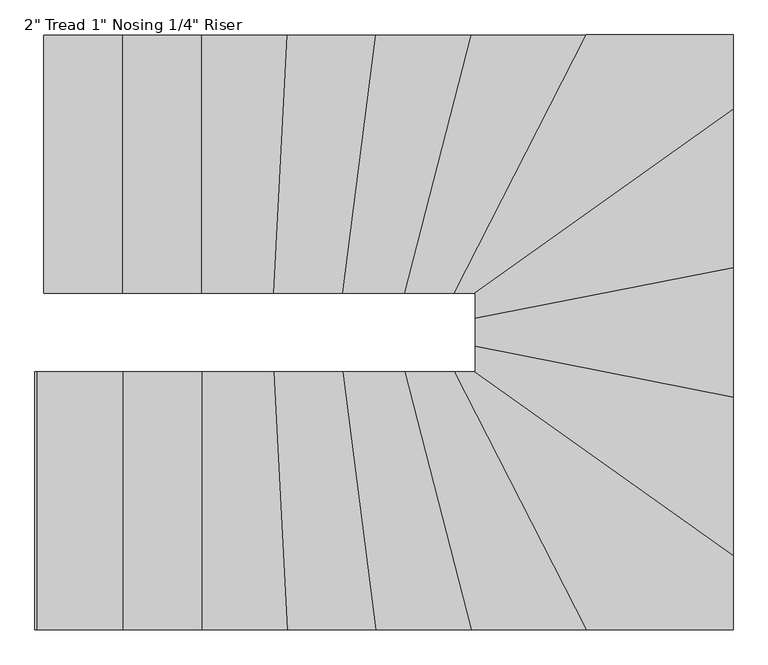
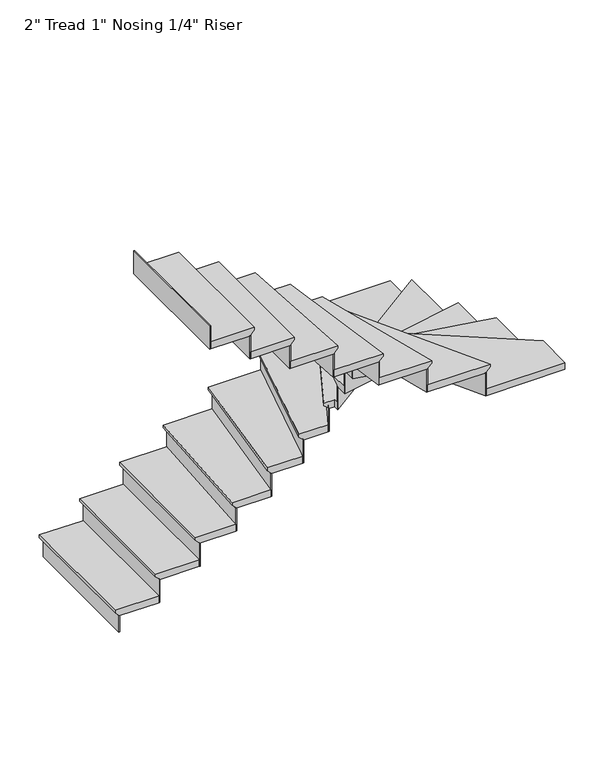
"""IFC4 building model written with IfcOpenShell, lengths in millimetres: stair flight geometry."""

from ifc_helpers import new_model, si_unit, origin, place, context, project, spatial, faceted_brep, source, transform, mapped, element, save


def stair_flight_0756a42a(model_context):
    return source(origin(), model_context, "Body", "Brep", [
        faceted_brep([(306.9570026, -4376.7064015, 3350.6833333), (306.9570026, -4376.7064015, 3369.7333333), (306.9570026, -3462.3064015, 3369.7333333), (306.9570026, -3462.3064015, 3350.6833333), (332.3570026, -4376.7064015, 3325.2833333), (332.3570026, -3462.3064015, 3325.2833333), (611.7570026, -4376.7064015, 3369.7333333), (611.7570026, -3462.3064015, 3369.7333333), (332.3570026, -3462.3064015, 3318.9333333), (611.7570026, -3462.3064015, 3318.9333333), (611.7570026, -4376.7064015, 3318.9333333), (332.3570026, -4376.7064015, 3318.9333333)], [[[0, 1, 2, 3]], [[4, 0, 3, 5]], [[2, 1, 6, 7]], [[8, 9, 10, 11]], [[2, 7, 9, 8, 5, 3]], [[8, 11, 4, 5]], [[6, 1, 0, 4, 11, 10]], [[7, 6, 10, 9]]]),
        faceted_brep([(332.3570026, -4376.7064015, 3318.9333333), (332.3570026, -4376.7064015, 3200.4), (338.7070026, -4376.7064015, 3200.4), (338.7070026, -4376.7064015, 3318.9333333), (332.3570026, -3462.3064015, 3318.9333333), (338.7070026, -3462.3064015, 3318.9333333), (338.7070026, -3462.3064015, 3200.4), (332.3570026, -3462.3064015, 3200.4)], [[[0, 1, 2, 3]], [[4, 5, 6, 7]], [[1, 0, 4, 7]], [[2, 1, 7, 6]], [[3, 2, 6, 5]], [[0, 3, 5, 4]]]),
        faceted_brep([(611.7570026, -4376.7064015, 3488.2666667), (611.7570026, -4376.7064015, 3318.9333333), (618.1070026, -4376.7064015, 3318.9333333), (618.1070026, -4376.7064015, 3488.2666667), (611.7570026, -3462.3064015, 3488.2666667), (618.1070026, -3462.3064015, 3488.2666667), (618.1070026, -3462.3064015, 3318.9333333), (611.7570026, -3462.3064015, 3318.9333333)], [[[0, 1, 2, 3]], [[4, 5, 6, 7]], [[1, 0, 4, 7]], [[2, 1, 7, 6]], [[3, 2, 6, 5]], [[0, 3, 5, 4]]]),
        faceted_brep([(586.3570026, -3462.3064015, 3539.0666667), (586.3570026, -4376.7064015, 3539.0666667), (891.1570026, -4376.7064015, 3539.0666667), (891.1570026, -3462.3064015, 3539.0666667), (611.7570026, -3462.3064015, 3488.2666667), (891.1570026, -3462.3064015, 3488.2666667), (891.1570026, -4376.7064015, 3488.2666667), (611.7570026, -4376.7064015, 3488.2666667), (611.7570026, -3462.3064015, 3494.6166667), (586.3570026, -3462.3064015, 3520.0166667), (611.7570026, -4376.7064015, 3494.6166667), (586.3570026, -4376.7064015, 3520.0166667)], [[[0, 1, 2, 3]], [[4, 5, 6, 7]], [[0, 3, 5, 4, 8, 9]], [[4, 7, 10, 8]], [[2, 1, 11, 10, 7, 6]], [[3, 2, 6, 5]], [[11, 1, 0, 9]], [[10, 11, 9, 8]]]),
        faceted_brep([(891.1570026, -4376.7064015, 3657.6), (891.1570026, -4376.7064015, 3488.2666667), (897.5070026, -4376.7064015, 3488.2666667), (897.5070026, -4376.7064015, 3657.6), (891.1570026, -3462.3064015, 3657.6), (897.5070026, -3462.3064015, 3657.6), (897.5070026, -3462.3064015, 3488.2666667), (891.1570026, -3462.3064015, 3488.2666667)], [[[0, 1, 2, 3]], [[4, 5, 6, 7]], [[1, 0, 4, 7]], [[2, 1, 7, 6]], [[3, 2, 6, 5]], [[0, 3, 5, 4]]]),
        faceted_brep([(865.7570026, -3462.3064015, 3708.4), (865.7570026, -4376.7064015, 3708.4), (1146.824164, -4376.7064015, 3708.4), (1194.3584344, -3462.3064015, 3708.4), (891.1570026, -3462.3064015, 3657.6), (1194.3584344, -3462.3064015, 3657.6), (1146.824164, -4376.7064015, 3657.6), (891.1570026, -4376.7064015, 3657.6), (891.1570026, -3462.3064015, 3663.95), (865.7570026, -3462.3064015, 3689.35), (891.1570026, -4376.7064015, 3663.95), (865.7570026, -4376.7064015, 3689.35)], [[[0, 1, 2, 3]], [[4, 5, 6, 7]], [[0, 3, 5, 4, 8, 9]], [[4, 7, 10, 8]], [[2, 1, 11, 10, 7, 6]], [[3, 2, 6, 5]], [[11, 1, 0, 9]], [[10, 11, 9, 8]]]),
        faceted_brep([(1146.824164, -4376.7064015, 3826.9333333), (1146.824164, -4376.7064015, 3657.6), (1153.1827382, -4376.7064015, 3657.6), (1153.1827382, -4376.7064015, 3826.9333333), (1194.3584344, -3462.3064015, 3826.9333333), (1200.7170086, -3462.3064015, 3826.9333333), (1200.7170086, -3462.3064015, 3657.6), (1194.3584344, -3462.3064015, 3657.6)], [[[0, 1, 2, 3]], [[4, 5, 6, 7]], [[1, 0, 4, 7]], [[2, 1, 7, 6]], [[3, 2, 6, 5]], [[0, 3, 5, 4]]]),
        faceted_brep([(1168.9241378, -3462.3064015, 3877.7333333), (1121.3898673, -4376.7064015, 3877.7333333), (1390.9908638, -4376.7064015, 3877.7333333), (1509.3469155, -3462.3064015, 3877.7333333), (1194.3584344, -3462.3064015, 3826.9333333), (1509.3469155, -3462.3064015, 3826.9333333), (1390.9908638, -4376.7064015, 3826.9333333), (1146.824164, -4376.7064015, 3826.9333333), (1194.3584344, -3462.3064015, 3833.2833333), (1168.9241378, -3462.3064015, 3858.6833333), (1146.824164, -4376.7064015, 3833.2833333), (1121.3898673, -4376.7064015, 3858.6833333)], [[[0, 1, 2, 3]], [[4, 5, 6, 7]], [[0, 3, 5, 4, 8, 9]], [[4, 7, 10, 8]], [[2, 1, 11, 10, 7, 6]], [[3, 2, 6, 5]], [[11, 1, 0, 9]], [[10, 11, 9, 8]]]),
        faceted_brep([(1390.9908638, -4376.7064015, 3996.2666667), (1390.9908638, -4376.7064015, 3826.9333333), (1397.3938356, -4376.7064015, 3826.9333333), (1397.3938356, -4376.7064015, 3996.2666667), (1509.3469155, -3462.3064015, 3996.2666667), (1515.7498873, -3462.3064015, 3996.2666667), (1515.7498873, -3462.3064015, 3826.9333333), (1509.3469155, -3462.3064015, 3826.9333333)], [[[0, 1, 2, 3]], [[4, 5, 6, 7]], [[1, 0, 4, 7]], [[2, 1, 7, 6]], [[3, 2, 6, 5]], [[0, 3, 5, 4]]]),
        faceted_brep([(1483.7350284, -3462.3064015, 4047.0666667), (1365.3789767, -4376.7064015, 4047.0666667), (1612.6180863, -4376.7064015, 4047.0666667), (1847.7485337, -3462.3064015, 4047.0666667), (1509.3469155, -3462.3064015, 3996.2666667), (1847.7485337, -3462.3064015, 3996.2666667), (1612.6180863, -4376.7064015, 3996.2666667), (1390.9908638, -4376.7064015, 3996.2666667), (1509.3469155, -3462.3064015, 4002.6166667), (1483.7350284, -3462.3064015, 4028.0166667), (1390.9908638, -4376.7064015, 4002.6166667), (1365.3789767, -4376.7064015, 4028.0166667)], [[[0, 1, 2, 3]], [[4, 5, 6, 7]], [[0, 3, 5, 4, 8, 9]], [[4, 7, 10, 8]], [[2, 1, 11, 10, 7, 6]], [[3, 2, 6, 5]], [[11, 1, 0, 9]], [[10, 11, 9, 8]]]),
        faceted_brep([(1612.6180863, -4376.7064015, 4165.6), (1612.6180863, -4376.7064015, 3996.2666667), (1619.1746632, -4376.7064015, 3996.2666667), (1619.1746632, -4376.7064015, 4165.6), (1847.7485337, -3462.3064015, 4165.6), (1854.3051106, -3462.3064015, 4165.6), (1854.3051106, -3462.3064015, 3996.2666667), (1847.7485337, -3462.3064015, 3996.2666667)], [[[0, 1, 2, 3]], [[4, 5, 6, 7]], [[1, 0, 4, 7]], [[2, 1, 7, 6]], [[3, 2, 6, 5]], [[0, 3, 5, 4]]]),
        faceted_brep([(1821.5222263, -3462.3064015, 4216.4), (1586.3917788, -4376.7064015, 4216.4), (1788.9647224, -4376.7064015, 4216.4), (2257.7893437, -3462.3064015, 4216.4), (1847.7485337, -3462.3064015, 4165.6), (2257.7893437, -3462.3064015, 4165.6), (1788.9647224, -4376.7064015, 4165.6), (1612.6180863, -4376.7064015, 4165.6), (1847.7485337, -3462.3064015, 4171.95), (1821.5222263, -3462.3064015, 4197.35), (1612.6180863, -4376.7064015, 4171.95), (1586.3917788, -4376.7064015, 4197.35)], [[[0, 1, 2, 3]], [[4, 5, 6, 7]], [[0, 3, 5, 4, 8, 9]], [[4, 7, 10, 8]], [[2, 1, 11, 10, 7, 6]], [[3, 2, 6, 5]], [[11, 1, 0, 9]], [[10, 11, 9, 8]]]),
        faceted_brep([(1788.9647224, -4376.7064015, 4334.9333333), (1788.9647224, -4376.7064015, 4165.6), (1796.1007055, -4376.7064015, 4165.6), (1796.1007055, -4376.7064015, 4334.9333333), (2257.7893437, -3462.3064015, 4334.9333333), (2264.9253269, -3462.3064015, 4334.9333333), (2264.9253269, -3462.3064015, 4165.6), (2257.7893437, -3462.3064015, 4165.6)], [[[0, 1, 2, 3]], [[4, 5, 6, 7]], [[1, 0, 4, 7]], [[2, 1, 7, 6]], [[3, 2, 6, 5]], [[0, 3, 5, 4]]]),
        faceted_brep([(2749.0886944, -3755.9875352, 4385.7333333), (2749.0886944, -3462.3064015, 4385.7333333), (2229.2454112, -3462.3064015, 4385.7333333), (1760.4207899, -4376.7064015, 4385.7333333), (1834.6886944, -4376.7064015, 4385.7333333), (1834.6886944, -4406.2614844, 4385.7333333), (2749.0886944, -3462.3064015, 4334.9333333), (2749.0886944, -3755.9875352, 4334.9333333), (1834.6886944, -4406.2614844, 4334.9333333), (1834.6886944, -4376.7064015, 4334.9333333), (1788.9647224, -4376.7064015, 4334.9333333), (2257.7893437, -3462.3064015, 4334.9333333), (2257.7893437, -3462.3064015, 4341.2833333), (2229.2454112, -3462.3064015, 4366.6833333), (1788.9647224, -4376.7064015, 4341.2833333), (1760.4207899, -4376.7064015, 4366.6833333)], [[[0, 1, 2, 3, 4, 5]], [[6, 7, 8, 9, 10, 11]], [[1, 0, 7, 6]], [[2, 1, 6, 11, 12, 13]], [[11, 10, 14, 12]], [[4, 3, 15, 14, 10, 9]], [[5, 4, 9, 8]], [[0, 5, 8, 7]], [[15, 3, 2, 13]], [[14, 15, 13, 12]]]),
        faceted_brep([(1834.6886944, -4406.2614844, 4504.2666667), (1834.6886944, -4406.2614844, 4334.9333333), (1834.6886944, -4414.0534592, 4334.9333333), (1834.6886944, -4414.0534592, 4504.2666667), (2749.0886944, -3755.9875352, 4504.2666667), (2749.0886944, -3763.77951, 4504.2666667), (2749.0886944, -3763.77951, 4334.9333333), (2749.0886944, -3755.9875352, 4334.9333333)], [[[0, 1, 2, 3]], [[4, 5, 6, 7]], [[1, 0, 4, 7]], [[2, 1, 7, 6]], [[3, 2, 6, 5]], [[0, 3, 5, 4]]]),
        faceted_brep([(2749.0886944, -3724.819636, 4555.0666667), (1834.6886944, -4375.0935852, 4555.0666667), (1834.6886944, -4492.7155714, 4555.0666667), (2749.0886944, -4312.4747151, 4555.0666667), (2749.0886944, -3755.9875352, 4504.2666667), (2749.0886944, -4312.4747151, 4504.2666667), (1834.6886944, -4492.7155714, 4504.2666667), (1834.6886944, -4406.2614844, 4504.2666667), (2749.0886944, -3755.9875352, 4510.6166667), (2749.0886944, -3724.819636, 4536.0166667), (1834.6886944, -4406.2614844, 4510.6166667), (1834.6886944, -4375.0935852, 4536.0166667)], [[[0, 1, 2, 3]], [[4, 5, 6, 7]], [[0, 3, 5, 4, 8, 9]], [[4, 7, 10, 8]], [[2, 1, 11, 10, 7, 6]], [[3, 2, 6, 5]], [[11, 1, 0, 9]], [[10, 11, 9, 8]]]),
        faceted_brep([(1834.6886944, -4492.7155714, 4673.6), (1834.6886944, -4492.7155714, 4504.2666667), (1834.6886944, -4499.1877569, 4504.2666667), (1834.6886944, -4499.1877569, 4673.6), (2749.0886944, -4312.4747151, 4673.6), (2749.0886944, -4318.9469005, 4673.6), (2749.0886944, -4318.9469005, 4504.2666667), (2749.0886944, -4312.4747151, 4504.2666667)], [[[0, 1, 2, 3]], [[4, 5, 6, 7]], [[1, 0, 4, 7]], [[2, 1, 7, 6]], [[3, 2, 6, 5]], [[0, 3, 5, 4]]]),
        faceted_brep([(2749.0886944, -4286.5859733, 4724.4), (1834.6886944, -4466.8268297, 4724.4), (1834.6886944, -4591.8747151, 4724.4), (2749.0886944, -4772.1155714, 4724.4), (2749.0886944, -4312.4747151, 4673.6), (2749.0886944, -4772.1155714, 4673.6), (1834.6886944, -4591.8747151, 4673.6), (1834.6886944, -4492.7155714, 4673.6), (2749.0886944, -4312.4747151, 4679.95), (2749.0886944, -4286.5859733, 4705.35), (1834.6886944, -4492.7155714, 4679.95), (1834.6886944, -4466.8268297, 4705.35)], [[[0, 1, 2, 3]], [[4, 5, 6, 7]], [[0, 3, 5, 4, 8, 9]], [[4, 7, 10, 8]], [[2, 1, 11, 10, 7, 6]], [[3, 2, 6, 5]], [[11, 1, 0, 9]], [[10, 11, 9, 8]]]),
        faceted_brep([(1834.6886944, -4591.8747151, 4842.9333333), (1834.6886944, -4591.8747151, 4673.6), (1834.6886944, -4598.3469005, 4673.6), (1834.6886944, -4598.3469005, 4842.9333333), (2749.0886944, -4772.1155714, 4842.9333333), (2749.0886944, -4778.5877569, 4842.9333333), (2749.0886944, -4778.5877569, 4673.6), (2749.0886944, -4772.1155714, 4673.6)], [[[0, 1, 2, 3]], [[4, 5, 6, 7]], [[1, 0, 4, 7]], [[2, 1, 7, 6]], [[3, 2, 6, 5]], [[0, 3, 5, 4]]]),
        faceted_brep([(2749.0886944, -4746.2268297, 4893.7333333), (1834.6886944, -4565.9859733, 4893.7333333), (1834.6886944, -4656.1064015, 4893.7333333), (1788.5932199, -4656.1064015, 4893.7333333), (2749.0886944, -5339.1610662, 4893.7333333), (2749.0886944, -4772.1155714, 4842.9333333), (2749.0886944, -5339.1610662, 4842.9333333), (1788.5932199, -4656.1064015, 4842.9333333), (1834.6886944, -4656.1064015, 4842.9333333), (1834.6886944, -4591.8747151, 4842.9333333), (2749.0886944, -4772.1155714, 4849.2833333), (2749.0886944, -4746.2268297, 4874.6833333), (1834.6886944, -4591.8747151, 4849.2833333), (1834.6886944, -4565.9859733, 4874.6833333)], [[[0, 1, 2, 3, 4]], [[5, 6, 7, 8, 9]], [[0, 4, 6, 5, 10, 11]], [[5, 9, 12, 10]], [[2, 1, 13, 12, 9, 8]], [[3, 2, 8, 7]], [[4, 3, 7, 6]], [[13, 1, 0, 11]], [[12, 13, 11, 10]]]),
        faceted_brep([(1788.5932199, -4656.1064015, 5012.2666667), (1788.5932199, -4656.1064015, 4842.9333333), (1777.6363274, -4656.1064015, 4842.9333333), (1777.6363274, -4656.1064015, 5012.2666667), (2749.0886944, -5339.1610662, 5012.2666667), (2749.0886944, -5346.953041, 5012.2666667), (2749.0886944, -5346.953041, 4842.9333333), (2749.0886944, -5339.1610662, 4842.9333333)], [[[0, 1, 2, 3]], [[4, 5, 6, 7]], [[1, 0, 4, 7]], [[2, 1, 7, 6]], [[3, 2, 6, 5]], [[0, 3, 5, 4]]]),
        faceted_brep([(2200.7014787, -5570.5064015, 5063.0666667), (2749.0886944, -5570.5064015, 5063.0666667), (2749.0886944, -5307.993167, 5063.0666667), (1832.4207899, -4656.1064015, 5063.0666667), (1731.8768573, -4656.1064015, 5063.0666667), (2749.0886944, -5570.5064015, 5012.2666667), (2200.7014787, -5570.5064015, 5012.2666667), (1731.8768573, -4656.1064015, 5012.2666667), (1788.5932199, -4656.1064015, 5012.2666667), (2749.0886944, -5339.1610662, 5012.2666667), (2749.0886944, -5339.1610662, 5018.6166667), (2749.0886944, -5307.993167, 5044.0166667), (1788.5932199, -4656.1064015, 5018.6166667), (1832.4207899, -4656.1064015, 5044.0166667)], [[[0, 1, 2, 3, 4]], [[5, 6, 7, 8, 9]], [[1, 0, 6, 5]], [[2, 1, 5, 9, 10, 11]], [[9, 8, 12, 10]], [[4, 3, 13, 12, 8, 7]], [[0, 4, 7, 6]], [[13, 3, 2, 11]], [[12, 13, 11, 10]]]),
        faceted_brep([(1731.8768573, -4656.1064015, 5181.6), (1731.8768573, -4656.1064015, 5012.2666667), (1724.7408742, -4656.1064015, 5012.2666667), (1724.7408742, -4656.1064015, 5181.6), (2200.7014787, -5570.5064015, 5181.6), (2193.5654955, -5570.5064015, 5181.6), (2193.5654955, -5570.5064015, 5012.2666667), (2200.7014787, -5570.5064015, 5012.2666667)], [[[0, 1, 2, 3]], [[4, 5, 6, 7]], [[1, 0, 4, 7]], [[2, 1, 7, 6]], [[3, 2, 6, 5]], [[0, 3, 5, 4]]]),
        faceted_brep([(2229.2454112, -5570.5064015, 5232.4), (1760.4207899, -4656.1064015, 5232.4), (1560.1654714, -4656.1064015, 5232.4), (1795.2959188, -5570.5064015, 5232.4), (2200.7014787, -5570.5064015, 5181.6), (1795.2959188, -5570.5064015, 5181.6), (1560.1654714, -4656.1064015, 5181.6), (1731.8768573, -4656.1064015, 5181.6), (2200.7014787, -5570.5064015, 5187.95), (2229.2454112, -5570.5064015, 5213.35), (1731.8768573, -4656.1064015, 5187.95), (1760.4207899, -4656.1064015, 5213.35)], [[[0, 1, 2, 3]], [[4, 5, 6, 7]], [[0, 3, 5, 4, 8, 9]], [[4, 7, 10, 8]], [[2, 1, 11, 10, 7, 6]], [[3, 2, 6, 5]], [[11, 1, 0, 9]], [[10, 11, 9, 8]]]),
        faceted_brep([(1560.1654714, -4656.1064015, 5350.9333333), (1560.1654714, -4656.1064015, 5181.6), (1553.6088945, -4656.1064015, 5181.6), (1553.6088945, -4656.1064015, 5350.9333333), (1795.2959188, -5570.5064015, 5350.9333333), (1788.7393419, -5570.5064015, 5350.9333333), (1788.7393419, -5570.5064015, 5181.6), (1795.2959188, -5570.5064015, 5181.6)], [[[0, 1, 2, 3]], [[4, 5, 6, 7]], [[1, 0, 4, 7]], [[2, 1, 7, 6]], [[3, 2, 6, 5]], [[0, 3, 5, 4]]]),
        faceted_brep([(1821.5222263, -5570.5064015, 5401.7333333), (1586.3917788, -4656.1064015, 5401.7333333), (1339.7670896, -4656.1064015, 5401.7333333), (1458.1231413, -5570.5064015, 5401.7333333), (1795.2959188, -5570.5064015, 5350.9333333), (1458.1231413, -5570.5064015, 5350.9333333), (1339.7670896, -4656.1064015, 5350.9333333), (1560.1654714, -4656.1064015, 5350.9333333), (1795.2959188, -5570.5064015, 5357.2833333), (1821.5222263, -5570.5064015, 5382.6833333), (1560.1654714, -4656.1064015, 5357.2833333), (1586.3917788, -4656.1064015, 5382.6833333)], [[[0, 1, 2, 3]], [[4, 5, 6, 7]], [[0, 3, 5, 4, 8, 9]], [[4, 7, 10, 8]], [[2, 1, 11, 10, 7, 6]], [[3, 2, 6, 5]], [[11, 1, 0, 9]], [[10, 11, 9, 8]]]),
        faceted_brep([(1339.7670896, -4656.1064015, 5520.2666667), (1339.7670896, -4656.1064015, 5350.9333333), (1333.3641178, -4656.1064015, 5350.9333333), (1333.3641178, -4656.1064015, 5520.2666667), (1458.1231413, -5570.5064015, 5520.2666667), (1451.7201695, -5570.5064015, 5520.2666667), (1451.7201695, -5570.5064015, 5350.9333333), (1458.1231413, -5570.5064015, 5350.9333333)], [[[0, 1, 2, 3]], [[4, 5, 6, 7]], [[1, 0, 4, 7]], [[2, 1, 7, 6]], [[3, 2, 6, 5]], [[0, 3, 5, 4]]]),
        faceted_brep([(1483.7350284, -5570.5064015, 5571.0666667), (1365.3789767, -4656.1064015, 5571.0666667), (1095.9555707, -4656.1064015, 5571.0666667), (1143.4898411, -5570.5064015, 5571.0666667), (1458.1231413, -5570.5064015, 5520.2666667), (1143.4898411, -5570.5064015, 5520.2666667), (1095.9555707, -4656.1064015, 5520.2666667), (1339.7670896, -4656.1064015, 5520.2666667), (1458.1231413, -5570.5064015, 5526.6166667), (1483.7350284, -5570.5064015, 5552.0166667), (1339.7670896, -4656.1064015, 5526.6166667), (1365.3789767, -4656.1064015, 5552.0166667)], [[[0, 1, 2, 3]], [[4, 5, 6, 7]], [[0, 3, 5, 4, 8, 9]], [[4, 7, 10, 8]], [[2, 1, 11, 10, 7, 6]], [[3, 2, 6, 5]], [[11, 1, 0, 9]], [[10, 11, 9, 8]]]),
        faceted_brep([(1095.9555707, -4656.1064015, 5689.6), (1095.9555707, -4656.1064015, 5520.2666667), (1089.5969965, -4656.1064015, 5520.2666667), (1089.5969965, -4656.1064015, 5689.6), (1143.4898411, -5570.5064015, 5689.6), (1137.1312669, -5570.5064015, 5689.6), (1137.1312669, -5570.5064015, 5520.2666667), (1143.4898411, -5570.5064015, 5520.2666667)], [[[0, 1, 2, 3]], [[4, 5, 6, 7]], [[1, 0, 4, 7]], [[2, 1, 7, 6]], [[3, 2, 6, 5]], [[0, 3, 5, 4]]]),
        faceted_brep([(1168.9241378, -5570.5064015, 5740.4), (1121.3898673, -4656.1064015, 5740.4), (840.3570026, -4656.1064015, 5740.4), (840.3570026, -5570.5064015, 5740.4), (1143.4898411, -5570.5064015, 5689.6), (840.3570026, -5570.5064015, 5689.6), (840.3570026, -4656.1064015, 5689.6), (1095.9555707, -4656.1064015, 5689.6), (1143.4898411, -5570.5064015, 5695.95), (1168.9241378, -5570.5064015, 5721.35), (1095.9555707, -4656.1064015, 5695.95), (1121.3898673, -4656.1064015, 5721.35)], [[[0, 1, 2, 3]], [[4, 5, 6, 7]], [[0, 3, 5, 4, 8, 9]], [[4, 7, 10, 8]], [[2, 1, 11, 10, 7, 6]], [[3, 2, 6, 5]], [[11, 1, 0, 9]], [[10, 11, 9, 8]]]),
        faceted_brep([(840.3570026, -4656.1064015, 5858.9333333), (840.3570026, -4656.1064015, 5689.6), (834.0070026, -4656.1064015, 5689.6), (834.0070026, -4656.1064015, 5858.9333333), (840.3570026, -5570.5064015, 5858.9333333), (834.0070026, -5570.5064015, 5858.9333333), (834.0070026, -5570.5064015, 5689.6), (840.3570026, -5570.5064015, 5689.6)], [[[0, 1, 2, 3]], [[4, 5, 6, 7]], [[1, 0, 4, 7]], [[2, 1, 7, 6]], [[3, 2, 6, 5]], [[0, 3, 5, 4]]]),
        faceted_brep([(865.7570026, -5570.5064015, 5909.7333333), (865.7570026, -4656.1064015, 5909.7333333), (560.9570026, -4656.1064015, 5909.7333333), (560.9570026, -5570.5064015, 5909.7333333), (840.3570026, -5570.5064015, 5858.9333333), (560.9570026, -5570.5064015, 5858.9333333), (560.9570026, -4656.1064015, 5858.9333333), (840.3570026, -4656.1064015, 5858.9333333), (840.3570026, -5570.5064015, 5865.2833333), (865.7570026, -5570.5064015, 5890.6833333), (840.3570026, -4656.1064015, 5865.2833333), (865.7570026, -4656.1064015, 5890.6833333)], [[[0, 1, 2, 3]], [[4, 5, 6, 7]], [[0, 3, 5, 4, 8, 9]], [[4, 7, 10, 8]], [[2, 1, 11, 10, 7, 6]], [[3, 2, 6, 5]], [[11, 1, 0, 9]], [[10, 11, 9, 8]]]),
        faceted_brep([(560.9570026, -4656.1064015, 6028.2666667), (560.9570026, -4656.1064015, 5858.9333333), (554.6070026, -4656.1064015, 5858.9333333), (554.6070026, -4656.1064015, 6028.2666667), (560.9570026, -5570.5064015, 6028.2666667), (554.6070026, -5570.5064015, 6028.2666667), (554.6070026, -5570.5064015, 5858.9333333), (560.9570026, -5570.5064015, 5858.9333333)], [[[0, 1, 2, 3]], [[4, 5, 6, 7]], [[1, 0, 4, 7]], [[2, 1, 7, 6]], [[3, 2, 6, 5]], [[0, 3, 5, 4]]]),
        faceted_brep([(281.5570026, -4656.1064015, 6197.6), (281.5570026, -4656.1064015, 6028.2666667), (275.2070026, -4656.1064015, 6028.2666667), (275.2070026, -4656.1064015, 6197.6), (281.5570026, -5570.5064015, 6197.6), (275.2070026, -5570.5064015, 6197.6), (275.2070026, -5570.5064015, 6028.2666667), (281.5570026, -5570.5064015, 6028.2666667)], [[[0, 1, 2, 3]], [[4, 5, 6, 7]], [[1, 0, 4, 7]], [[2, 1, 7, 6]], [[3, 2, 6, 5]], [[0, 3, 5, 4]]]),
        faceted_brep([(586.3570026, -5570.5064015, 6079.0666667), (586.3570026, -4656.1064015, 6079.0666667), (281.5570026, -4656.1064015, 6079.0666667), (281.5570026, -5570.5064015, 6079.0666667), (560.9570026, -5570.5064015, 6028.2666667), (281.5570026, -5570.5064015, 6028.2666667), (281.5570026, -4656.1064015, 6028.2666667), (560.9570026, -4656.1064015, 6028.2666667), (560.9570026, -5570.5064015, 6034.6166667), (586.3570026, -5570.5064015, 6060.0166667), (560.9570026, -4656.1064015, 6034.6166667), (586.3570026, -4656.1064015, 6060.0166667)], [[[0, 1, 2, 3]], [[4, 5, 6, 7]], [[0, 3, 5, 4, 8, 9]], [[4, 7, 10, 8]], [[2, 1, 11, 10, 7, 6]], [[3, 2, 6, 5]], [[11, 1, 0, 9]], [[10, 11, 9, 8]]]),
    ])


if __name__ == "__main__":
    model = new_model("IFC4")
    model_context = context("Model", 3, world=origin())
    ifc_project = project(units=[si_unit("LENGTHUNIT", "METRE", prefix="MILLI")], contexts=[model_context])
    site = spatial("IfcSite", under=ifc_project)
    building = spatial("IfcBuilding", under=site)
    placement = place(None, origin())
    stair_flight_shape = stair_flight_0756a42a(model_context)
    element("IfcStairFlight", 1, ObjectType="2\" Tread 1\" Nosing 1/4\" Riser", at=placement, inside=building, context=model_context, shape_type="MappedRepresentation", body=[
        mapped(stair_flight_shape, transform((0.0, 0.0, 0.0), x_axis=(1.0, 0.0, 0.0), y_axis=(0.0, 1.0, 0.0), z_axis=(0.0, 0.0, 1.0))),
    ])
    save(model, "model.ifc")
